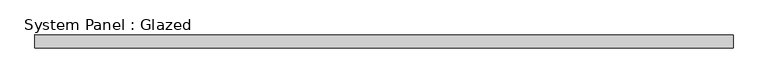
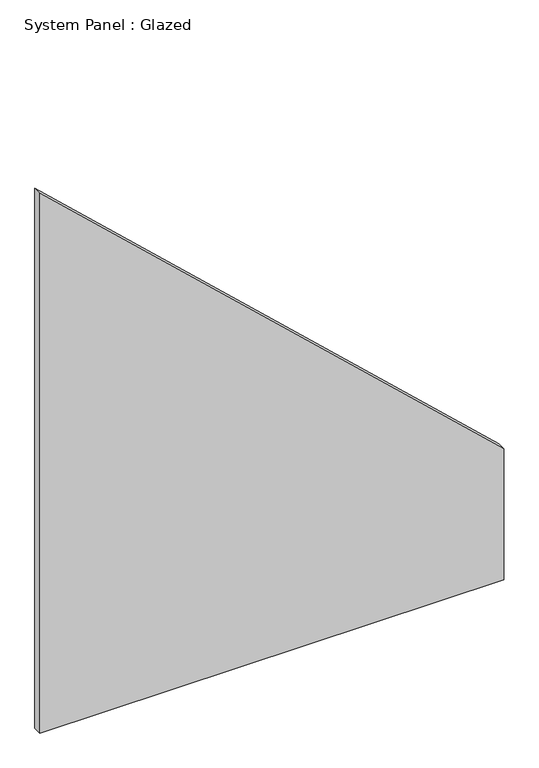
"""IFC4 building model written with IfcOpenShell, lengths in millimetres: plate geometry, System Panel : Glazed."""

from ifc_helpers import new_model, si_unit, frame, origin, place, context, project, spatial, polyline, outline, extrude, source, transform, mapped, element, save


def system_panel_glazed_b4bfdf73(model_context):
    return source(origin(), model_context, "Body", "SweptSolid", [
        extrude(outline(polyline([(0.0, -675.6150228), (0.0, 675.6150228), (402.3044798, 675.6150228), (1662.3468822, -675.6150228), (0.0, -675.6150228)])), frame((0.0, 19.05, 0.0), z_axis=(0.0, 1.0, 0.0), x_axis=(0.0, 0.0, 1.0)), (0.0, 0.0, 1.0), 25.4),
    ])


if __name__ == "__main__":
    model = new_model("IFC4")
    model_context = context("Model", 3, world=origin())
    ifc_project = project(units=[si_unit("LENGTHUNIT", "METRE", prefix="MILLI")], contexts=[model_context])
    site = spatial("IfcSite", under=ifc_project)
    building = spatial("IfcBuilding", under=site)
    placement = place(None, origin())
    system_panel_glazed_shape = system_panel_glazed_b4bfdf73(model_context)
    element("IfcPlate", 1, ObjectType="System Panel : Glazed", at=placement, inside=building, context=model_context, shape_type="MappedRepresentation", body=[
        mapped(system_panel_glazed_shape, transform((0.0, 0.0, 0.0), x_axis=(1.0, 0.0, 0.0), y_axis=(0.0, 1.0, 0.0), z_axis=(0.0, 0.0, 1.0))),
    ])
    save(model, "model.ifc")

# Revit data of these elements
# Type "System Panel : Glazed"
#   Construction Type Id = "GSP4R"
#   Analytic Construction = "1/8 in Pilkington single glazing"
#   Visual Light Transmittance = 0.9
#   Solar Heat Gain Coefficient = 0.86
#   Heat Transfer Coefficient (U) = 1.18115 BTU/(h·ft²·°F)
#   Define Thermal Properties by = 1
# Element 1 (IfcPlate, "System Panel : Glazed")
#   Materials on its faces: "Glass"
# Materials
#   "Glass": class "Glass", colour RGB 0 128 192, transparency 0.75, Description = "Soda Lime Glass", Cost = 0
